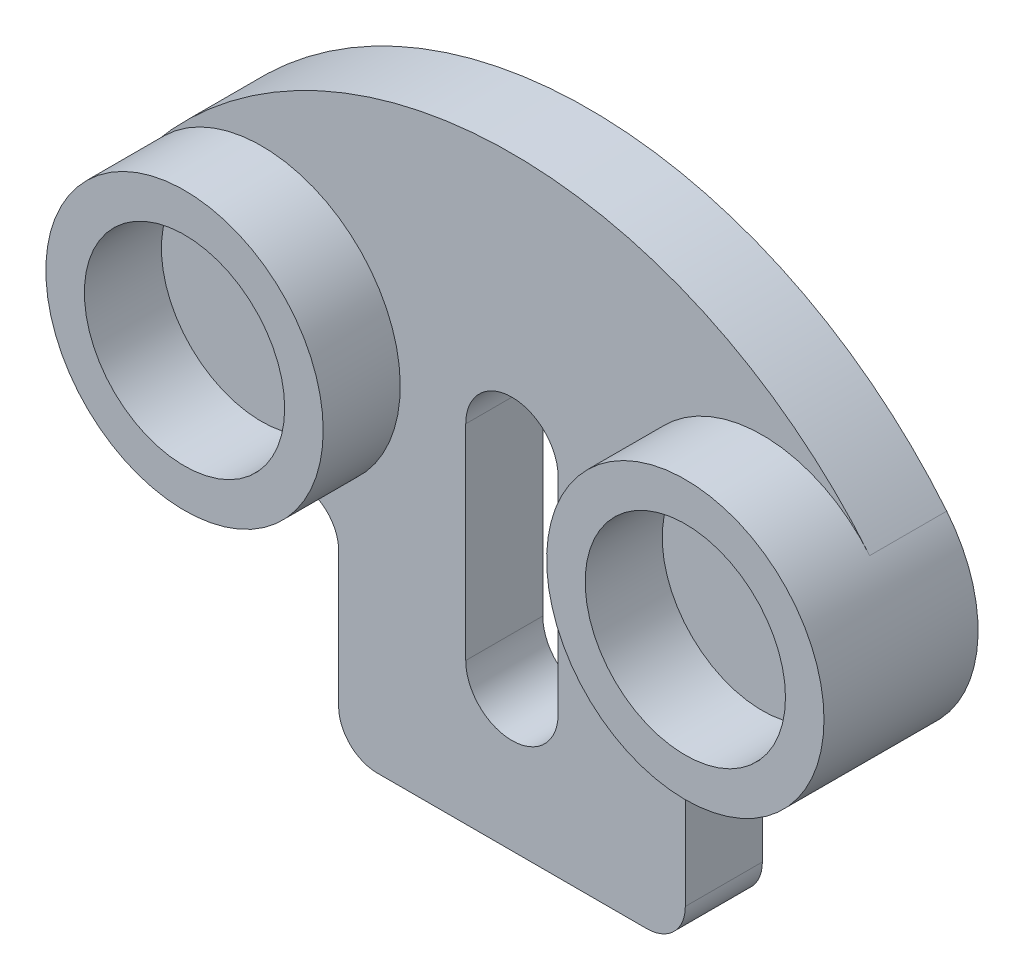
ISO-10303-21;
HEADER;
FILE_DESCRIPTION(('STEP AP214'),'2;1');
FILE_NAME('part.step','',(''),(''),'','','');
FILE_SCHEMA(('AUTOMOTIVE_DESIGN { 1 0 10303 214 1 1 1 1 }'));
ENDSEC;
DATA;
#1=APPLICATION_CONTEXT('core data for automotive mechanical design processes');
#2=APPLICATION_PROTOCOL_DEFINITION('international standard','automotive_design',2000,#1);
#3=PRODUCT_CONTEXT('',#1,'mechanical');
#4=PRODUCT('Part','Part','',(#3));
#5=PRODUCT_RELATED_PRODUCT_CATEGORY('part','',(#4));
#6=PRODUCT_DEFINITION_FORMATION('','',#4);
#7=PRODUCT_DEFINITION_CONTEXT('part definition',#1,'design');
#8=PRODUCT_DEFINITION('design','',#6,#7);
#9=PRODUCT_DEFINITION_SHAPE('','',#8);
#10=(LENGTH_UNIT() NAMED_UNIT(*) SI_UNIT(.MILLI.,.METRE.));
#11=(NAMED_UNIT(*) PLANE_ANGLE_UNIT() SI_UNIT($,.RADIAN.));
#12=(NAMED_UNIT(*) SI_UNIT($,.STERADIAN.) SOLID_ANGLE_UNIT());
#13=UNCERTAINTY_MEASURE_WITH_UNIT(LENGTH_MEASURE(1.E-05),#10,'distance_accuracy_value','');
#14=(GEOMETRIC_REPRESENTATION_CONTEXT(3) GLOBAL_UNCERTAINTY_ASSIGNED_CONTEXT((#13)) GLOBAL_UNIT_ASSIGNED_CONTEXT((#10,
#11,#12)) REPRESENTATION_CONTEXT('',''));
#15=CARTESIAN_POINT('',(0.,0.,0.));
#16=DIRECTION('',(0.,0.,1.));
#17=DIRECTION('',(1.,0.,0.));
#18=AXIS2_PLACEMENT_3D('',#15,#16,#17);
#19=CARTESIAN_POINT('',(0.,26.6035711888461,10.));
#20=DIRECTION('',(0.,0.,-1.));
#21=DIRECTION('',(-1.,0.,0.));
#22=AXIS2_PLACEMENT_3D('',#19,#20,#21);
#23=CYLINDRICAL_SURFACE('',#22,6.);
#24=CARTESIAN_POINT('',(0.,26.6035711888461,0.));
#25=DIRECTION('',(0.,0.,1.));
#26=DIRECTION('',(1.,0.,0.));
#27=AXIS2_PLACEMENT_3D('',#24,#25,#26);
#28=CIRCLE('',#27,6.);
#29=CARTESIAN_POINT('',(6.,26.6035711888461,0.));
#30=VERTEX_POINT('',#29);
#31=CARTESIAN_POINT('',(-6.,26.6035711888461,0.));
#32=VERTEX_POINT('',#31);
#33=EDGE_CURVE('E253',#30,#32,#28,.T.);
#34=ORIENTED_EDGE('',*,*,#33,.F.);
#35=DIRECTION('',(0.,0.,-1.));
#36=VECTOR('',#35,1.);
#37=CARTESIAN_POINT('',(6.,26.6035711888461,10.));
#38=LINE('',#37,#36);
#39=CARTESIAN_POINT('',(6.,26.6035711888461,10.));
#40=VERTEX_POINT('',#39);
#41=EDGE_CURVE('E220',#40,#30,#38,.T.);
#42=ORIENTED_EDGE('',*,*,#41,.F.);
#43=CARTESIAN_POINT('',(0.,26.6035711888461,10.));
#44=DIRECTION('',(0.,0.,1.));
#45=DIRECTION('',(1.,0.,0.));
#46=AXIS2_PLACEMENT_3D('',#43,#44,#45);
#47=CIRCLE('',#46,6.);
#48=CARTESIAN_POINT('',(-6.,26.6035711888461,10.));
#49=VERTEX_POINT('',#48);
#50=EDGE_CURVE('E210',#40,#49,#47,.T.);
#51=ORIENTED_EDGE('',*,*,#50,.T.);
#52=DIRECTION('',(0.,0.,-1.));
#53=VECTOR('',#52,1.);
#54=CARTESIAN_POINT('',(-6.,26.6035711888461,10.));
#55=LINE('',#54,#53);
#56=EDGE_CURVE('E122',#49,#32,#55,.T.);
#57=ORIENTED_EDGE('',*,*,#56,.T.);
#58=EDGE_LOOP('',(#34,#42,#51,#57));
#59=FACE_BOUND('',#58,.T.);
#60=ADVANCED_FACE('F110',(#59),#23,.F.);
#61=CARTESIAN_POINT('',(6.,0.,10.));
#62=DIRECTION('',(1.,0.,0.));
#63=DIRECTION('',(0.,0.,-1.));
#64=AXIS2_PLACEMENT_3D('',#61,#62,#63);
#65=PLANE('',#64);
#66=DIRECTION('',(0.,-1.,0.));
#67=VECTOR('',#66,1.);
#68=CARTESIAN_POINT('',(6.,0.,0.));
#69=LINE('',#68,#67);
#70=CARTESIAN_POINT('',(6.,0.,0.));
#71=VERTEX_POINT('',#70);
#72=EDGE_CURVE('E212',#30,#71,#69,.T.);
#73=ORIENTED_EDGE('',*,*,#72,.T.);
#74=DIRECTION('',(0.,0.,-1.));
#75=VECTOR('',#74,1.);
#76=CARTESIAN_POINT('',(6.,0.,10.));
#77=LINE('',#76,#75);
#78=CARTESIAN_POINT('',(6.,0.,10.));
#79=VERTEX_POINT('',#78);
#80=EDGE_CURVE('E211',#79,#71,#77,.T.);
#81=ORIENTED_EDGE('',*,*,#80,.F.);
#82=DIRECTION('',(0.,-1.,0.));
#83=VECTOR('',#82,1.);
#84=CARTESIAN_POINT('',(6.,0.,10.));
#85=LINE('',#84,#83);
#86=EDGE_CURVE('E203',#40,#79,#85,.T.);
#87=ORIENTED_EDGE('',*,*,#86,.F.);
#88=ORIENTED_EDGE('',*,*,#41,.T.);
#89=EDGE_LOOP('',(#73,#81,#87,#88));
#90=FACE_BOUND('',#89,.T.);
#91=ADVANCED_FACE('F215',(#90),#65,.F.);
#92=CARTESIAN_POINT('',(0.,0.,10.));
#93=DIRECTION('',(0.,0.,-1.));
#94=DIRECTION('',(-1.,0.,0.));
#95=AXIS2_PLACEMENT_3D('',#92,#93,#94);
#96=CYLINDRICAL_SURFACE('',#95,6.);
#97=CARTESIAN_POINT('',(0.,0.,0.));
#98=DIRECTION('',(0.,0.,1.));
#99=DIRECTION('',(1.,0.,0.));
#100=AXIS2_PLACEMENT_3D('',#97,#98,#99);
#101=CIRCLE('',#100,6.);
#102=CARTESIAN_POINT('',(-6.,0.,0.));
#103=VERTEX_POINT('',#102);
#104=EDGE_CURVE('E255',#103,#71,#101,.T.);
#105=ORIENTED_EDGE('',*,*,#104,.F.);
#106=DIRECTION('',(0.,0.,-1.));
#107=VECTOR('',#106,1.);
#108=CARTESIAN_POINT('',(-6.,0.,10.));
#109=LINE('',#108,#107);
#110=CARTESIAN_POINT('',(-6.,0.,10.));
#111=VERTEX_POINT('',#110);
#112=EDGE_CURVE('E162',#111,#103,#109,.T.);
#113=ORIENTED_EDGE('',*,*,#112,.F.);
#114=CARTESIAN_POINT('',(0.,0.,10.));
#115=DIRECTION('',(0.,0.,1.));
#116=DIRECTION('',(1.,0.,0.));
#117=AXIS2_PLACEMENT_3D('',#114,#115,#116);
#118=CIRCLE('',#117,6.);
#119=EDGE_CURVE('E206',#111,#79,#118,.T.);
#120=ORIENTED_EDGE('',*,*,#119,.T.);
#121=ORIENTED_EDGE('',*,*,#80,.T.);
#122=EDGE_LOOP('',(#105,#113,#120,#121));
#123=FACE_BOUND('',#122,.T.);
#124=ADVANCED_FACE('F218',(#123),#96,.F.);
#125=CARTESIAN_POINT('',(-17.5,-13.3964288111539,10.));
#126=DIRECTION('',(0.,0.,-1.));
#127=DIRECTION('',(-1.,0.,0.));
#128=AXIS2_PLACEMENT_3D('',#125,#126,#127);
#129=CYLINDRICAL_SURFACE('',#128,5.);
#130=CARTESIAN_POINT('',(-17.5,-13.3964288111539,0.));
#131=DIRECTION('',(0.,0.,1.));
#132=DIRECTION('',(1.,0.,0.));
#133=AXIS2_PLACEMENT_3D('',#130,#131,#132);
#134=CIRCLE('',#133,5.);
#135=CARTESIAN_POINT('',(-17.5,-18.3964288111539,0.));
#136=VERTEX_POINT('',#135);
#137=CARTESIAN_POINT('',(-22.5,-13.3964288111539,0.));
#138=VERTEX_POINT('',#137);
#139=EDGE_CURVE('E229',#136,#138,#134,.F.);
#140=ORIENTED_EDGE('',*,*,#139,.F.);
#141=DIRECTION('',(0.,0.,-1.));
#142=VECTOR('',#141,1.);
#143=CARTESIAN_POINT('',(-17.5,-18.3964288111539,10.));
#144=LINE('',#143,#142);
#145=CARTESIAN_POINT('',(-17.5,-18.3964288111539,10.));
#146=VERTEX_POINT('',#145);
#147=EDGE_CURVE('E172',#146,#136,#144,.T.);
#148=ORIENTED_EDGE('',*,*,#147,.F.);
#149=CARTESIAN_POINT('',(-17.5,-13.3964288111539,10.));
#150=DIRECTION('',(0.,0.,1.));
#151=DIRECTION('',(1.,0.,0.));
#152=AXIS2_PLACEMENT_3D('',#149,#150,#151);
#153=CIRCLE('',#152,5.);
#154=CARTESIAN_POINT('',(-22.5,-13.3964288111539,10.));
#155=VERTEX_POINT('',#154);
#156=EDGE_CURVE('E259',#146,#155,#153,.F.);
#157=ORIENTED_EDGE('',*,*,#156,.T.);
#158=DIRECTION('',(0.,0.,-1.));
#159=VECTOR('',#158,1.);
#160=CARTESIAN_POINT('',(-22.5,-13.3964288111539,10.));
#161=LINE('',#160,#159);
#162=EDGE_CURVE('E225',#155,#138,#161,.T.);
#163=ORIENTED_EDGE('',*,*,#162,.T.);
#164=EDGE_LOOP('',(#140,#148,#157,#163));
#165=FACE_BOUND('',#164,.T.);
#166=ADVANCED_FACE('F108',(#165),#129,.T.);
#167=CARTESIAN_POINT('',(0.,-18.3964288111539,10.));
#168=DIRECTION('',(0.,1.,0.));
#169=DIRECTION('',(0.,0.,1.));
#170=AXIS2_PLACEMENT_3D('',#167,#168,#169);
#171=PLANE('',#170);
#172=DIRECTION('',(1.,0.,0.));
#173=VECTOR('',#172,1.);
#174=CARTESIAN_POINT('',(0.,-18.3964288111539,0.));
#175=LINE('',#174,#173);
#176=CARTESIAN_POINT('',(17.5,-18.3964288111539,0.));
#177=VERTEX_POINT('',#176);
#178=EDGE_CURVE('E228',#136,#177,#175,.T.);
#179=ORIENTED_EDGE('',*,*,#178,.T.);
#180=DIRECTION('',(0.,0.,-1.));
#181=VECTOR('',#180,1.);
#182=CARTESIAN_POINT('',(17.5,-18.3964288111539,10.));
#183=LINE('',#182,#181);
#184=CARTESIAN_POINT('',(17.5,-18.3964288111539,10.));
#185=VERTEX_POINT('',#184);
#186=EDGE_CURVE('E281',#185,#177,#183,.T.);
#187=ORIENTED_EDGE('',*,*,#186,.F.);
#188=DIRECTION('',(1.,0.,0.));
#189=VECTOR('',#188,1.);
#190=CARTESIAN_POINT('',(0.,-18.3964288111539,10.));
#191=LINE('',#190,#189);
#192=EDGE_CURVE('E313',#146,#185,#191,.T.);
#193=ORIENTED_EDGE('',*,*,#192,.F.);
#194=ORIENTED_EDGE('',*,*,#147,.T.);
#195=EDGE_LOOP('',(#179,#187,#193,#194));
#196=FACE_BOUND('',#195,.T.);
#197=ADVANCED_FACE('F374',(#196),#171,.F.);
#198=CARTESIAN_POINT('',(17.5,-13.3964288111539,10.));
#199=DIRECTION('',(0.,0.,-1.));
#200=DIRECTION('',(-1.,0.,0.));
#201=AXIS2_PLACEMENT_3D('',#198,#199,#200);
#202=CYLINDRICAL_SURFACE('',#201,5.);
#203=CARTESIAN_POINT('',(17.5,-13.3964288111539,0.));
#204=DIRECTION('',(0.,0.,1.));
#205=DIRECTION('',(1.,0.,0.));
#206=AXIS2_PLACEMENT_3D('',#203,#204,#205);
#207=CIRCLE('',#206,5.);
#208=CARTESIAN_POINT('',(22.5,-13.3964288111539,0.));
#209=VERTEX_POINT('',#208);
#210=EDGE_CURVE('E233',#209,#177,#207,.F.);
#211=ORIENTED_EDGE('',*,*,#210,.F.);
#212=DIRECTION('',(0.,0.,-1.));
#213=VECTOR('',#212,1.);
#214=CARTESIAN_POINT('',(22.5,-13.3964288111539,10.));
#215=LINE('',#214,#213);
#216=CARTESIAN_POINT('',(22.5,-13.3964288111539,10.));
#217=VERTEX_POINT('',#216);
#218=EDGE_CURVE('E278',#217,#209,#215,.T.);
#219=ORIENTED_EDGE('',*,*,#218,.F.);
#220=CARTESIAN_POINT('',(17.5,-13.3964288111539,10.));
#221=DIRECTION('',(0.,0.,1.));
#222=DIRECTION('',(1.,0.,0.));
#223=AXIS2_PLACEMENT_3D('',#220,#221,#222);
#224=CIRCLE('',#223,5.);
#225=EDGE_CURVE('E311',#217,#185,#224,.F.);
#226=ORIENTED_EDGE('',*,*,#225,.T.);
#227=ORIENTED_EDGE('',*,*,#186,.T.);
#228=EDGE_LOOP('',(#211,#219,#226,#227));
#229=FACE_BOUND('',#228,.T.);
#230=ADVANCED_FACE('F375',(#229),#202,.T.);
#231=CARTESIAN_POINT('',(22.5,0.,10.));
#232=DIRECTION('',(-1.,0.,0.));
#233=DIRECTION('',(0.,-1.,0.));
#234=AXIS2_PLACEMENT_3D('',#231,#232,#233);
#235=PLANE('',#234);
#236=DIRECTION('',(0.,1.,0.));
#237=VECTOR('',#236,1.);
#238=CARTESIAN_POINT('',(22.5,0.,0.));
#239=LINE('',#238,#237);
#240=CARTESIAN_POINT('',(22.5,4.1536268682024,0.));
#241=VERTEX_POINT('',#240);
#242=EDGE_CURVE('E237',#209,#241,#239,.T.);
#243=ORIENTED_EDGE('',*,*,#242,.T.);
#244=DIRECTION('',(0.,0.,-1.));
#245=VECTOR('',#244,1.);
#246=CARTESIAN_POINT('',(22.5,4.1536268682024,10.));
#247=LINE('',#246,#245);
#248=CARTESIAN_POINT('',(22.5,4.1536268682024,10.));
#249=VERTEX_POINT('',#248);
#250=EDGE_CURVE('E279',#249,#241,#247,.T.);
#251=ORIENTED_EDGE('',*,*,#250,.F.);
#252=DIRECTION('',(0.,1.,0.));
#253=VECTOR('',#252,1.);
#254=CARTESIAN_POINT('',(22.5,0.,10.));
#255=LINE('',#254,#253);
#256=EDGE_CURVE('E316',#217,#249,#255,.T.);
#257=ORIENTED_EDGE('',*,*,#256,.F.);
#258=ORIENTED_EDGE('',*,*,#218,.T.);
#259=EDGE_LOOP('',(#243,#251,#257,#258));
#260=FACE_BOUND('',#259,.T.);
#261=ADVANCED_FACE('F366',(#260),#235,.F.);
#262=CARTESIAN_POINT('',(27.5,4.1536268682024,10.));
#263=DIRECTION('',(0.,0.,-1.));
#264=DIRECTION('',(-1.,0.,0.));
#265=AXIS2_PLACEMENT_3D('',#262,#263,#264);
#266=CYLINDRICAL_SURFACE('',#265,5.);
#267=CARTESIAN_POINT('',(27.5,4.1536268682024,0.));
#268=DIRECTION('',(0.,0.,1.));
#269=DIRECTION('',(1.,0.,0.));
#270=AXIS2_PLACEMENT_3D('',#267,#268,#269);
#271=CIRCLE('',#270,5.);
#272=CARTESIAN_POINT('',(28.5869565217391,9.03404954660319,0.));
#273=VERTEX_POINT('',#272);
#274=EDGE_CURVE('E239',#273,#241,#271,.T.);
#275=ORIENTED_EDGE('',*,*,#274,.F.);
#276=DIRECTION('',(0.,0.,-1.));
#277=VECTOR('',#276,1.);
#278=CARTESIAN_POINT('',(28.5869565217391,9.03404954660319,10.));
#279=LINE('',#278,#277);
#280=CARTESIAN_POINT('',(28.5869565217391,9.03404954660319,10.));
#281=VERTEX_POINT('',#280);
#282=EDGE_CURVE('E274',#281,#273,#279,.T.);
#283=ORIENTED_EDGE('',*,*,#282,.F.);
#284=CARTESIAN_POINT('',(27.5,4.1536268682024,10.));
#285=DIRECTION('',(0.,0.,1.));
#286=DIRECTION('',(1.,0.,0.));
#287=AXIS2_PLACEMENT_3D('',#284,#285,#286);
#288=CIRCLE('',#287,5.);
#289=EDGE_CURVE('E318',#281,#249,#288,.T.);
#290=ORIENTED_EDGE('',*,*,#289,.T.);
#291=ORIENTED_EDGE('',*,*,#250,.T.);
#292=EDGE_LOOP('',(#275,#283,#290,#291));
#293=FACE_BOUND('',#292,.T.);
#294=ADVANCED_FACE('F364',(#293),#266,.F.);
#295=CARTESIAN_POINT('',(0.,0.,10.));
#296=DIRECTION('',(0.,0.,-1.));
#297=DIRECTION('',(-1.,0.,0.));
#298=AXIS2_PLACEMENT_3D('',#295,#296,#297);
#299=CYLINDRICAL_SURFACE('',#298,60.);
#300=CARTESIAN_POINT('',(0.,0.,0.));
#301=DIRECTION('',(0.,0.,1.));
#302=DIRECTION('',(1.,0.,0.));
#303=AXIS2_PLACEMENT_3D('',#300,#301,#302);
#304=CIRCLE('',#303,60.);
#305=CARTESIAN_POINT('',(46.4285714285714,38.0051016983515,0.));
#306=VERTEX_POINT('',#305);
#307=CARTESIAN_POINT('',(-46.4285714285714,38.0051016983515,0.));
#308=VERTEX_POINT('',#307);
#309=EDGE_CURVE('E241',#306,#308,#304,.T.);
#310=ORIENTED_EDGE('',*,*,#309,.T.);
#311=DIRECTION('',(0.,0.,-1.));
#312=VECTOR('',#311,1.);
#313=CARTESIAN_POINT('',(-46.4285714285714,38.0051016983515,10.));
#314=LINE('',#313,#312);
#315=CARTESIAN_POINT('',(-46.4285714285714,38.0051016983515,10.));
#316=VERTEX_POINT('',#315);
#317=EDGE_CURVE('E267',#316,#308,#314,.T.);
#318=ORIENTED_EDGE('',*,*,#317,.F.);
#319=CARTESIAN_POINT('',(0.,0.,10.));
#320=DIRECTION('',(0.,0.,1.));
#321=DIRECTION('',(1.,0.,0.));
#322=AXIS2_PLACEMENT_3D('',#319,#320,#321);
#323=CIRCLE('',#322,60.);
#324=CARTESIAN_POINT('',(46.4285714285714,38.0051016983515,10.));
#325=VERTEX_POINT('',#324);
#326=EDGE_CURVE('E322',#325,#316,#323,.T.);
#327=ORIENTED_EDGE('',*,*,#326,.F.);
#328=DIRECTION('',(0.,0.,-1.));
#329=VECTOR('',#328,1.);
#330=CARTESIAN_POINT('',(46.4285714285714,38.0051016983515,10.));
#331=LINE('',#330,#329);
#332=EDGE_CURVE('E275',#325,#306,#331,.T.);
#333=ORIENTED_EDGE('',*,*,#332,.T.);
#334=EDGE_LOOP('',(#310,#318,#327,#333));
#335=FACE_BOUND('',#334,.T.);
#336=ADVANCED_FACE('F363',(#335),#299,.T.);
#337=CARTESIAN_POINT('',(-27.5,4.1536268682024,10.));
#338=DIRECTION('',(0.,0.,-1.));
#339=DIRECTION('',(-1.,0.,0.));
#340=AXIS2_PLACEMENT_3D('',#337,#338,#339);
#341=CYLINDRICAL_SURFACE('',#340,5.);
#342=CARTESIAN_POINT('',(-27.5,4.1536268682024,0.));
#343=DIRECTION('',(0.,0.,1.));
#344=DIRECTION('',(1.,0.,0.));
#345=AXIS2_PLACEMENT_3D('',#342,#343,#344);
#346=CIRCLE('',#345,5.);
#347=CARTESIAN_POINT('',(-22.5,4.1536268682024,0.));
#348=VERTEX_POINT('',#347);
#349=CARTESIAN_POINT('',(-28.5869565217391,9.0340495466032,0.));
#350=VERTEX_POINT('',#349);
#351=EDGE_CURVE('E242',#348,#350,#346,.T.);
#352=ORIENTED_EDGE('',*,*,#351,.F.);
#353=DIRECTION('',(0.,0.,-1.));
#354=VECTOR('',#353,1.);
#355=CARTESIAN_POINT('',(-22.5,4.1536268682024,10.));
#356=LINE('',#355,#354);
#357=CARTESIAN_POINT('',(-22.5,4.1536268682024,10.));
#358=VERTEX_POINT('',#357);
#359=EDGE_CURVE('E262',#358,#348,#356,.T.);
#360=ORIENTED_EDGE('',*,*,#359,.F.);
#361=CARTESIAN_POINT('',(-27.5,4.1536268682024,10.));
#362=DIRECTION('',(0.,0.,1.));
#363=DIRECTION('',(1.,0.,0.));
#364=AXIS2_PLACEMENT_3D('',#361,#362,#363);
#365=CIRCLE('',#364,5.);
#366=CARTESIAN_POINT('',(-28.5869565217391,9.0340495466032,10.));
#367=VERTEX_POINT('',#366);
#368=EDGE_CURVE('E329',#358,#367,#365,.T.);
#369=ORIENTED_EDGE('',*,*,#368,.T.);
#370=DIRECTION('',(0.,0.,-1.));
#371=VECTOR('',#370,1.);
#372=CARTESIAN_POINT('',(-28.5869565217391,9.03404954660319,10.));
#373=LINE('',#372,#371);
#374=EDGE_CURVE('E266',#367,#350,#373,.T.);
#375=ORIENTED_EDGE('',*,*,#374,.T.);
#376=EDGE_LOOP('',(#352,#360,#369,#375));
#377=FACE_BOUND('',#376,.T.);
#378=ADVANCED_FACE('F350',(#377),#341,.F.);
#379=CARTESIAN_POINT('',(-22.5,0.,10.));
#380=DIRECTION('',(-1.,0.,0.));
#381=DIRECTION('',(0.,0.,1.));
#382=AXIS2_PLACEMENT_3D('',#379,#380,#381);
#383=PLANE('',#382);
#384=DIRECTION('',(0.,1.,0.));
#385=VECTOR('',#384,1.);
#386=CARTESIAN_POINT('',(-22.5,0.,0.));
#387=LINE('',#386,#385);
#388=EDGE_CURVE('E248',#138,#348,#387,.T.);
#389=ORIENTED_EDGE('',*,*,#388,.F.);
#390=ORIENTED_EDGE('',*,*,#162,.F.);
#391=DIRECTION('',(0.,1.,0.));
#392=VECTOR('',#391,1.);
#393=CARTESIAN_POINT('',(-22.5,0.,10.));
#394=LINE('',#393,#392);
#395=EDGE_CURVE('E334',#155,#358,#394,.T.);
#396=ORIENTED_EDGE('',*,*,#395,.T.);
#397=ORIENTED_EDGE('',*,*,#359,.T.);
#398=EDGE_LOOP('',(#389,#390,#396,#397));
#399=FACE_BOUND('',#398,.T.);
#400=ADVANCED_FACE('F336',(#399),#383,.T.);
#401=CARTESIAN_POINT('',(-6.,0.,10.));
#402=DIRECTION('',(1.,0.,0.));
#403=DIRECTION('',(0.,0.,-1.));
#404=AXIS2_PLACEMENT_3D('',#401,#402,#403);
#405=PLANE('',#404);
#406=DIRECTION('',(0.,-1.,0.));
#407=VECTOR('',#406,1.);
#408=CARTESIAN_POINT('',(-6.,0.,0.));
#409=LINE('',#408,#407);
#410=EDGE_CURVE('E258',#32,#103,#409,.T.);
#411=ORIENTED_EDGE('',*,*,#410,.F.);
#412=ORIENTED_EDGE('',*,*,#56,.F.);
#413=DIRECTION('',(0.,-1.,0.));
#414=VECTOR('',#413,1.);
#415=CARTESIAN_POINT('',(-6.,0.,10.));
#416=LINE('',#415,#414);
#417=EDGE_CURVE('E219',#49,#111,#416,.T.);
#418=ORIENTED_EDGE('',*,*,#417,.T.);
#419=ORIENTED_EDGE('',*,*,#112,.T.);
#420=EDGE_LOOP('',(#411,#412,#418,#419));
#421=FACE_BOUND('',#420,.T.);
#422=ADVANCED_FACE('F333',(#421),#405,.T.);
#423=CARTESIAN_POINT('',(0.,0.,10.));
#424=DIRECTION('',(0.,0.,1.));
#425=DIRECTION('',(1.,0.,0.));
#426=AXIS2_PLACEMENT_3D('',#423,#424,#425);
#427=PLANE('',#426);
#428=ORIENTED_EDGE('',*,*,#156,.F.);
#429=ORIENTED_EDGE('',*,*,#192,.T.);
#430=ORIENTED_EDGE('',*,*,#225,.F.);
#431=ORIENTED_EDGE('',*,*,#256,.T.);
#432=ORIENTED_EDGE('',*,*,#289,.F.);
#433=CARTESIAN_POINT('',(32.5,26.6035711888461,10.));
#434=DIRECTION('',(0.,0.,1.));
#435=DIRECTION('',(1.,0.,0.));
#436=AXIS2_PLACEMENT_3D('',#433,#434,#435);
#437=CIRCLE('',#436,18.);
#438=EDGE_CURVE('E321',#325,#281,#437,.T.);
#439=ORIENTED_EDGE('',*,*,#438,.F.);
#440=ORIENTED_EDGE('',*,*,#326,.T.);
#441=CARTESIAN_POINT('',(-32.5,26.6035711888461,10.));
#442=DIRECTION('',(0.,0.,1.));
#443=DIRECTION('',(1.,0.,0.));
#444=AXIS2_PLACEMENT_3D('',#441,#442,#443);
#445=CIRCLE('',#444,18.);
#446=EDGE_CURVE('E330',#367,#316,#445,.T.);
#447=ORIENTED_EDGE('',*,*,#446,.F.);
#448=ORIENTED_EDGE('',*,*,#368,.F.);
#449=ORIENTED_EDGE('',*,*,#395,.F.);
#450=EDGE_LOOP('',(#428,#429,#430,#431,#432,#439,#440,#447,#448,#449));
#451=FACE_BOUND('',#450,.T.);
#452=ORIENTED_EDGE('',*,*,#50,.F.);
#453=ORIENTED_EDGE('',*,*,#86,.T.);
#454=ORIENTED_EDGE('',*,*,#119,.F.);
#455=ORIENTED_EDGE('',*,*,#417,.F.);
#456=EDGE_LOOP('',(#452,#453,#454,#455));
#457=FACE_BOUND('',#456,.T.);
#458=ADVANCED_FACE('F201',(#451,#457),#427,.T.);
#459=CARTESIAN_POINT('',(0.,0.,0.));
#460=DIRECTION('',(0.,0.,1.));
#461=DIRECTION('',(1.,0.,0.));
#462=AXIS2_PLACEMENT_3D('',#459,#460,#461);
#463=PLANE('',#462);
#464=ORIENTED_EDGE('',*,*,#139,.T.);
#465=ORIENTED_EDGE('',*,*,#388,.T.);
#466=ORIENTED_EDGE('',*,*,#351,.T.);
#467=CARTESIAN_POINT('',(-32.5,26.6035711888461,0.));
#468=DIRECTION('',(0.,0.,1.));
#469=DIRECTION('',(1.,0.,0.));
#470=AXIS2_PLACEMENT_3D('',#467,#468,#469);
#471=CIRCLE('',#470,18.);
#472=EDGE_CURVE('E298',#308,#350,#471,.T.);
#473=ORIENTED_EDGE('',*,*,#472,.F.);
#474=ORIENTED_EDGE('',*,*,#309,.F.);
#475=CARTESIAN_POINT('',(32.5,26.6035711888461,0.));
#476=DIRECTION('',(0.,0.,1.));
#477=DIRECTION('',(1.,0.,0.));
#478=AXIS2_PLACEMENT_3D('',#475,#476,#477);
#479=CIRCLE('',#478,18.);
#480=EDGE_CURVE('E307',#273,#306,#479,.T.);
#481=ORIENTED_EDGE('',*,*,#480,.F.);
#482=ORIENTED_EDGE('',*,*,#274,.T.);
#483=ORIENTED_EDGE('',*,*,#242,.F.);
#484=ORIENTED_EDGE('',*,*,#210,.T.);
#485=ORIENTED_EDGE('',*,*,#178,.F.);
#486=EDGE_LOOP('',(#464,#465,#466,#473,#474,#481,#482,#483,#484,#485));
#487=FACE_BOUND('',#486,.T.);
#488=ORIENTED_EDGE('',*,*,#33,.T.);
#489=ORIENTED_EDGE('',*,*,#410,.T.);
#490=ORIENTED_EDGE('',*,*,#104,.T.);
#491=ORIENTED_EDGE('',*,*,#72,.F.);
#492=EDGE_LOOP('',(#488,#489,#490,#491));
#493=FACE_BOUND('',#492,.T.);
#494=ADVANCED_FACE('F342',(#487,#493),#463,.F.);
#495=CARTESIAN_POINT('',(-32.5,26.6035711888461,20.));
#496=DIRECTION('',(0.,0.,-1.));
#497=DIRECTION('',(-1.,0.,0.));
#498=AXIS2_PLACEMENT_3D('',#495,#496,#497);
#499=CYLINDRICAL_SURFACE('',#498,18.);
#500=CARTESIAN_POINT('',(-32.5,26.6035711888461,20.));
#501=DIRECTION('',(0.,0.,1.));
#502=DIRECTION('',(1.,0.,0.));
#503=AXIS2_PLACEMENT_3D('',#500,#501,#502);
#504=CIRCLE('',#503,18.);
#505=CARTESIAN_POINT('',(-14.5,26.6035711888461,20.));
#506=VERTEX_POINT('',#505);
#507=EDGE_CURVE('E227',#506,#506,#504,.T.);
#508=ORIENTED_EDGE('',*,*,#507,.F.);
#509=EDGE_LOOP('',(#508));
#510=FACE_BOUND('',#509,.T.);
#511=ORIENTED_EDGE('',*,*,#446,.T.);
#512=ORIENTED_EDGE('',*,*,#317,.T.);
#513=ORIENTED_EDGE('',*,*,#472,.T.);
#514=ORIENTED_EDGE('',*,*,#374,.F.);
#515=EDGE_LOOP('',(#511,#512,#513,#514));
#516=FACE_BOUND('',#515,.T.);
#517=ADVANCED_FACE('F291',(#510,#516),#499,.T.);
#518=CARTESIAN_POINT('',(-32.5,26.6035711888461,20.));
#519=DIRECTION('',(0.,0.,-1.));
#520=DIRECTION('',(-1.,0.,0.));
#521=AXIS2_PLACEMENT_3D('',#518,#519,#520);
#522=CYLINDRICAL_SURFACE('',#521,13.);
#523=CARTESIAN_POINT('',(-32.5,26.6035711888461,10.));
#524=DIRECTION('',(0.,0.,1.));
#525=DIRECTION('',(1.,0.,0.));
#526=AXIS2_PLACEMENT_3D('',#523,#524,#525);
#527=CIRCLE('',#526,13.);
#528=CARTESIAN_POINT('',(-19.5,26.6035711888461,10.));
#529=VERTEX_POINT('',#528);
#530=EDGE_CURVE('E119',#529,#529,#527,.T.);
#531=ORIENTED_EDGE('',*,*,#530,.F.);
#532=EDGE_LOOP('',(#531));
#533=FACE_BOUND('',#532,.T.);
#534=CARTESIAN_POINT('',(-32.5,26.6035711888461,20.));
#535=DIRECTION('',(0.,0.,1.));
#536=DIRECTION('',(1.,0.,0.));
#537=AXIS2_PLACEMENT_3D('',#534,#535,#536);
#538=CIRCLE('',#537,13.);
#539=CARTESIAN_POINT('',(-19.5,26.6035711888461,20.));
#540=VERTEX_POINT('',#539);
#541=EDGE_CURVE('E296',#540,#540,#538,.T.);
#542=ORIENTED_EDGE('',*,*,#541,.T.);
#543=EDGE_LOOP('',(#542));
#544=FACE_BOUND('',#543,.T.);
#545=ADVANCED_FACE('F287',(#533,#544),#522,.F.);
#546=CARTESIAN_POINT('',(0.,0.,20.));
#547=DIRECTION('',(0.,0.,1.));
#548=DIRECTION('',(1.,0.,0.));
#549=AXIS2_PLACEMENT_3D('',#546,#547,#548);
#550=PLANE('',#549);
#551=ORIENTED_EDGE('',*,*,#541,.F.);
#552=EDGE_LOOP('',(#551));
#553=FACE_BOUND('',#552,.T.);
#554=ORIENTED_EDGE('',*,*,#507,.T.);
#555=EDGE_LOOP('',(#554));
#556=FACE_BOUND('',#555,.T.);
#557=ADVANCED_FACE('F295',(#553,#556),#550,.T.);
#558=CARTESIAN_POINT('',(0.,0.,10.));
#559=DIRECTION('',(0.,0.,1.));
#560=DIRECTION('',(1.,0.,0.));
#561=AXIS2_PLACEMENT_3D('',#558,#559,#560);
#562=PLANE('',#561);
#563=ORIENTED_EDGE('',*,*,#530,.T.);
#564=EDGE_LOOP('',(#563));
#565=FACE_BOUND('',#564,.T.);
#566=ADVANCED_FACE('F290',(#565),#562,.T.);
#567=CARTESIAN_POINT('',(32.5,26.6035711888461,20.));
#568=DIRECTION('',(0.,0.,-1.));
#569=DIRECTION('',(-1.,0.,0.));
#570=AXIS2_PLACEMENT_3D('',#567,#568,#569);
#571=CYLINDRICAL_SURFACE('',#570,18.);
#572=CARTESIAN_POINT('',(32.5,26.6035711888461,20.));
#573=DIRECTION('',(0.,0.,1.));
#574=DIRECTION('',(1.,0.,0.));
#575=AXIS2_PLACEMENT_3D('',#572,#573,#574);
#576=CIRCLE('',#575,18.);
#577=CARTESIAN_POINT('',(50.5,26.6035711888461,20.));
#578=VERTEX_POINT('',#577);
#579=EDGE_CURVE('E302',#578,#578,#576,.T.);
#580=ORIENTED_EDGE('',*,*,#579,.F.);
#581=EDGE_LOOP('',(#580));
#582=FACE_BOUND('',#581,.T.);
#583=ORIENTED_EDGE('',*,*,#438,.T.);
#584=ORIENTED_EDGE('',*,*,#282,.T.);
#585=ORIENTED_EDGE('',*,*,#480,.T.);
#586=ORIENTED_EDGE('',*,*,#332,.F.);
#587=EDGE_LOOP('',(#583,#584,#585,#586));
#588=FACE_BOUND('',#587,.T.);
#589=ADVANCED_FACE('F415',(#582,#588),#571,.T.);
#590=CARTESIAN_POINT('',(32.5,26.6035711888461,20.));
#591=DIRECTION('',(0.,0.,-1.));
#592=DIRECTION('',(-1.,0.,0.));
#593=AXIS2_PLACEMENT_3D('',#590,#591,#592);
#594=CYLINDRICAL_SURFACE('',#593,13.);
#595=CARTESIAN_POINT('',(32.5,26.6035711888461,10.));
#596=DIRECTION('',(0.,0.,1.));
#597=DIRECTION('',(1.,0.,0.));
#598=AXIS2_PLACEMENT_3D('',#595,#596,#597);
#599=CIRCLE('',#598,13.);
#600=CARTESIAN_POINT('',(45.5,26.6035711888461,10.));
#601=VERTEX_POINT('',#600);
#602=EDGE_CURVE('E12',#601,#601,#599,.T.);
#603=ORIENTED_EDGE('',*,*,#602,.F.);
#604=EDGE_LOOP('',(#603));
#605=FACE_BOUND('',#604,.T.);
#606=CARTESIAN_POINT('',(32.5,26.6035711888461,20.));
#607=DIRECTION('',(0.,0.,1.));
#608=DIRECTION('',(1.,0.,0.));
#609=AXIS2_PLACEMENT_3D('',#606,#607,#608);
#610=CIRCLE('',#609,13.);
#611=CARTESIAN_POINT('',(45.5,26.6035711888461,20.));
#612=VERTEX_POINT('',#611);
#613=EDGE_CURVE('E418',#612,#612,#610,.T.);
#614=ORIENTED_EDGE('',*,*,#613,.T.);
#615=EDGE_LOOP('',(#614));
#616=FACE_BOUND('',#615,.T.);
#617=ADVANCED_FACE('F435',(#605,#616),#594,.F.);
#618=CARTESIAN_POINT('',(0.,0.,20.));
#619=DIRECTION('',(0.,0.,1.));
#620=DIRECTION('',(1.,0.,0.));
#621=AXIS2_PLACEMENT_3D('',#618,#619,#620);
#622=PLANE('',#621);
#623=ORIENTED_EDGE('',*,*,#613,.F.);
#624=EDGE_LOOP('',(#623));
#625=FACE_BOUND('',#624,.T.);
#626=ORIENTED_EDGE('',*,*,#579,.T.);
#627=EDGE_LOOP('',(#626));
#628=FACE_BOUND('',#627,.T.);
#629=ADVANCED_FACE('F434',(#625,#628),#622,.T.);
#630=CARTESIAN_POINT('',(0.,0.,10.));
#631=DIRECTION('',(0.,0.,1.));
#632=DIRECTION('',(1.,0.,0.));
#633=AXIS2_PLACEMENT_3D('',#630,#631,#632);
#634=PLANE('',#633);
#635=ORIENTED_EDGE('',*,*,#602,.T.);
#636=EDGE_LOOP('',(#635));
#637=FACE_BOUND('',#636,.T.);
#638=ADVANCED_FACE('F445',(#637),#634,.T.);
#639=CLOSED_SHELL('',(#60,#91,#124,#166,#197,#230,#261,#294,#336,#378,#400,#422,#458,#494,#517,
#545,#557,#566,#589,#617,#629,#638));
#640=MANIFOLD_SOLID_BREP('B2',#639);
#641=ADVANCED_BREP_SHAPE_REPRESENTATION('',(#18,#640),#14);
#642=SHAPE_DEFINITION_REPRESENTATION(#9,#641);
ENDSEC;
END-ISO-10303-21;
